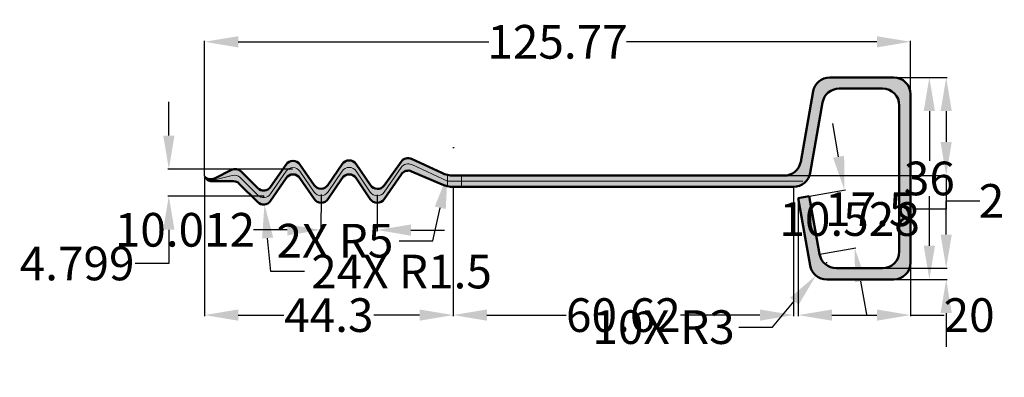
# Model space of a CAD drawing. Units: millimetres. Extents: x -64 to 111, y -49 to 15.
import ezdxf

# ---------------------------------------------------------------- set-up
doc = ezdxf.new("R2010")
doc.units = ezdxf.units.MM
doc.header["$MEASUREMENT"] = 0
doc.layers.add('M-DETL', color=251, linetype='Continuous', lineweight=18, true_color=0x636466)
doc.layers.add('M-HATC', color=251, linetype='Continuous', lineweight=18, true_color=0x636466)
doc.layers.add('M-DIMS', color=2, linetype='Continuous', lineweight=18)
doc.layers.add('M-OUTL', color=7, linetype='Continuous', lineweight=50)
doc.styles.get("Standard").update_dxf_attribs({"font": 'arial.ttf'})
doc.dimstyles.get("Standard").update_dxf_attribs({"dimtxt": 6, "dimasz": 6, "dimexe": 0.18, "dimexo": 0.0625, "dimgap": 0.09, "dimtad": 0, "dimtih": 1, "dimtoh": 1, "dimdec": 0, "dimzin": 0, "dimdsep": 46, "dimtxsty": 'Standard', "dimcen": 0.09, "dimadec": 0, "dimazin": 0, "dimtfac": 1, "dimtdec": 0, "dimtofl": 0, "dimtmove": 0, "dimatfit": 3, "dimfxl": 1, "dimtolj": 1, "dimtzin": 0, "dimarcsym": 0})

# ---------------------------------------------------------------- blocks, each defined once
blk = doc.blocks.new('*D1')
at = {"layer": 'Defpoints', "color": 0, "transparency": 16777216}
for p in [(94.41, 11.25), (94.41, 1.9), (-31.35, -12.77)]:
    blk.add_point(p, dxfattribs=at)
at = {"layer": 'M-DIMS', "color": 0, "lineweight": -2, "transparency": 16777216}
for p, q in [((-31.35, -12.71), (-31.35, 11.43)), ((-25.35, 11.25), (19.27, 11.25)), ((88.41, 11.25), (43.79, 11.25)), ((94.41, 1.97), (94.41, 11.43))]:
    blk.add_line(p, q, dxfattribs=at)
at = {"layer": 'M-DIMS', "color": 0, "transparency": 16777216}
for points in [[(-25.35, 12.25), (-25.35, 10.25), (-31.35, 11.25)], [(88.41, 12.25), (88.41, 10.25), (94.41, 11.25)]]:
    blk.add_solid(points, dxfattribs=at)
at = {"layer": 'M-DIMS', "color": 0, "transparency": 16777216, "insert": (31.53, 11.25), "char_height": 6, "attachment_point": 5}
blk.add_mtext('\\A1;125.77', dxfattribs=at)
blk = doc.blocks.new('*D2')
at = {"layer": 'Defpoints', "color": 0, "transparency": 16777216}
for p in [(91.41, 4.9), (91.41, -31.1), (97.76, -31.1)]:
    blk.add_point(p, dxfattribs=at)
at = {"layer": 'M-DIMS', "color": 0, "lineweight": -2, "transparency": 16777216}
for p, q in [((91.48, 4.9), (97.94, 4.9)), ((97.76, -1.1), (97.76, -9.94)), ((97.76, -25.1), (97.76, -16.25)), ((91.48, -31.1), (97.94, -31.1))]:
    blk.add_line(p, q, dxfattribs=at)
at = {"layer": 'M-DIMS', "color": 0, "transparency": 16777216}
for points in [[(96.76, -1.1), (98.76, -1.1), (97.76, 4.9)], [(96.76, -25.1), (98.76, -25.1), (97.76, -31.1)]]:
    blk.add_solid(points, dxfattribs=at)
at = {"layer": 'M-DIMS', "color": 0, "transparency": 16777216, "insert": (97.76, -13.1), "char_height": 6, "attachment_point": 5}
blk.add_mtext('\\A1;36', dxfattribs=at)
blk = doc.blocks.new('*D3')
at = {"layer": 'Defpoints', "color": 0, "transparency": 16777216}
for p in [(12.95, -14.6), (73.57, -14.6), (73.57, -37.45)]:
    blk.add_point(p, dxfattribs=at)
at = {"layer": 'M-DIMS', "color": 0, "lineweight": -2, "transparency": 16777216}
for p, q in [((12.95, -14.66), (12.95, -37.63)), ((73.57, -14.66), (73.57, -37.63)), ((18.95, -37.45), (33.06, -37.45)), ((67.57, -37.45), (53.46, -37.45))]:
    blk.add_line(p, q, dxfattribs=at)
at = {"layer": 'M-DIMS', "color": 0, "transparency": 16777216}
for points in [[(18.95, -36.45), (18.95, -38.45), (12.95, -37.45)], [(67.57, -36.45), (67.57, -38.45), (73.57, -37.45)]]:
    blk.add_solid(points, dxfattribs=at)
at = {"layer": 'M-DIMS', "color": 0, "transparency": 16777216, "insert": (43.26, -37.45), "char_height": 6, "attachment_point": 5}
blk.add_mtext('\\A1;60.62', dxfattribs=at)
blk = doc.blocks.new('*D4')
at = {"layer": 'Defpoints', "color": 0, "transparency": 16777216}
for p in [(74.41, -16.6), (94.41, -28.1), (94.41, -37.45)]:
    blk.add_point(p, dxfattribs=at)
at = {"layer": 'M-DIMS', "color": 0, "lineweight": -2, "transparency": 16777216}
for p, q in [((74.41, -16.66), (74.41, -37.63)), ((94.41, -28.16), (94.41, -37.63)), ((80.41, -37.45), (88.41, -37.45)), ((94.41, -37.45), (100.41, -37.45))]:
    blk.add_line(p, q, dxfattribs=at)
at = {"layer": 'M-DIMS', "color": 0, "transparency": 16777216}
for points in [[(80.41, -36.45), (80.41, -38.45), (74.41, -37.45)], [(88.41, -36.45), (88.41, -38.45), (94.41, -37.45)]]:
    blk.add_solid(points, dxfattribs=at)
at = {"layer": 'M-DIMS', "color": 0, "transparency": 16777216, "insert": (104.84, -37.45), "char_height": 6, "attachment_point": 5}
blk.add_mtext('\\A1;20', dxfattribs=at)
blk = doc.blocks.new('*D5')
at = {"layer": 'Defpoints', "color": 0, "transparency": 16777216}
for p in [(89.41, -29.1), (100.76, -29.1), (91.41, -31.1)]:
    blk.add_point(p, dxfattribs=at)
at = {"layer": 'M-DIMS', "color": 0, "lineweight": -2, "transparency": 16777216}
for p, q in [((100.76, -23.1), (100.76, -17.1)), ((100.76, -17.1), (106.76, -17.1)), ((89.48, -29.1), (100.94, -29.1)), ((91.48, -31.1), (100.94, -31.1)), ((100.76, -37.1), (100.76, -43.1))]:
    blk.add_line(p, q, dxfattribs=at)
at = {"layer": 'M-DIMS', "color": 0, "transparency": 16777216}
for points in [[(99.76, -23.1), (101.76, -23.1), (100.76, -29.1)], [(99.76, -37.1), (101.76, -37.1), (100.76, -31.1)]]:
    blk.add_solid(points, dxfattribs=at)
at = {"layer": 'M-DIMS', "color": 0, "transparency": 16777216, "insert": (108.84, -17.1), "char_height": 6, "attachment_point": 5}
blk.add_mtext('\\A1;2', dxfattribs=at)
blk = doc.blocks.new('*D6')
at = {"layer": 'Defpoints', "color": 0, "transparency": 16777216}
for p in [(91.41, 4.9), (71.9, -12.6), (100.76, -12.6)]:
    blk.add_point(p, dxfattribs=at)
at = {"layer": 'M-DIMS', "color": 0, "lineweight": -2, "transparency": 16777216}
for p, q in [((91.48, 4.9), (100.94, 4.9)), ((100.76, -1.1), (100.76, -6.6)), ((71.96, -12.6), (100.94, -12.6)), ((100.76, -12.6), (100.76, -18.6)), ((100.76, -18.6), (94.76, -18.6))]:
    blk.add_line(p, q, dxfattribs=at)
at = {"layer": 'M-DIMS', "color": 0, "transparency": 16777216}
for points in [[(99.76, -1.1), (101.76, -1.1), (100.76, 4.9)], [(99.76, -6.6), (101.76, -6.6), (100.76, -12.6)]]:
    blk.add_solid(points, dxfattribs=at)
at = {"layer": 'M-DIMS', "color": 0, "transparency": 16777216, "insert": (87.14, -18.6), "char_height": 6, "attachment_point": 5}
blk.add_mtext('\\A1;17.5', dxfattribs=at)
blk = doc.blocks.new('*D7')
at = {"layer": 'Defpoints', "color": 0, "transparency": 16777216}
for p in [(76.38, -16.25), (84.46, -25.51), (78.21, -26.62)]:
    blk.add_point(p, dxfattribs=at)
at = {"layer": 'M-DIMS', "color": 0, "lineweight": -2, "transparency": 16777216}
for p, q in [((81.59, -9.24), (80.55, -3.33)), ((76.44, -16.24), (82.81, -15.12)), ((78.27, -26.61), (84.64, -25.48)), ((85.51, -31.42), (86.55, -37.33))]:
    blk.add_line(p, q, dxfattribs=at)
at = {"layer": 'M-DIMS', "color": 0, "transparency": 16777216}
for points in [[(82.58, -9.06), (80.61, -9.41), (82.64, -15.15)], [(86.49, -31.25), (84.52, -31.6), (84.46, -25.51)]]:
    blk.add_solid(points, dxfattribs=at)
at = {"layer": 'M-DIMS', "color": 0, "transparency": 16777216, "insert": (83.55, -20.33), "char_height": 6, "attachment_point": 5}
blk.add_mtext('\\A1;10.528', dxfattribs=at)
blk = doc.blocks.new('*D8')
at = {"layer": 'Defpoints', "color": 0, "transparency": 16777216}
for p in [(-10.59, -15.92), (-0.57, -15.94), (-10.6, -22.27)]:
    blk.add_point(p, dxfattribs=at)
at = {"layer": 'M-DIMS', "color": 0, "lineweight": -2, "transparency": 16777216}
for p, q in [((-10.59, -15.98), (-10.6, -22.45)), ((-0.57, -16), (-0.59, -22.47)), ((-16.6, -22.26), (-22.6, -22.25)), ((5.41, -22.3), (11.41, -22.31))]:
    blk.add_line(p, q, dxfattribs=at)
at = {"layer": 'M-DIMS', "color": 0, "transparency": 16777216}
for points in [[(-16.6, -21.26), (-16.6, -23.26), (-10.6, -22.27)], [(5.42, -21.3), (5.41, -23.3), (-0.59, -22.29)]]:
    blk.add_solid(points, dxfattribs=at)
at = {"layer": 'M-DIMS', "color": 0, "transparency": 16777216, "insert": (-34.83, -22.25), "char_height": 6, "attachment_point": 5}
blk.add_mtext('\\A1;10.012', dxfattribs=at)
blk = doc.blocks.new('*D9')
at = {"layer": 'Defpoints', "color": 0, "transparency": 16777216}
for p in [(-31.35, -12.77), (12.95, -14.6), (12.95, -37.45)]:
    blk.add_point(p, dxfattribs=at)
at = {"layer": 'M-DIMS', "color": 0, "lineweight": -2, "transparency": 16777216}
for p, q in [((-31.35, -12.83), (-31.35, -37.63)), ((12.95, -14.66), (12.95, -37.63)), ((-25.35, -37.45), (-17.2, -37.45)), ((6.95, -37.45), (-1.2, -37.45))]:
    blk.add_line(p, q, dxfattribs=at)
at = {"layer": 'M-DIMS', "color": 0, "transparency": 16777216}
for points in [[(-25.35, -36.45), (-25.35, -38.45), (-31.35, -37.45)], [(6.95, -36.45), (6.95, -38.45), (12.95, -37.45)]]:
    blk.add_solid(points, dxfattribs=at)
at = {"layer": 'M-DIMS', "color": 0, "transparency": 16777216, "insert": (-9.2, -37.45), "char_height": 6, "attachment_point": 5}
blk.add_mtext('\\A1;44.3', dxfattribs=at)
blk = doc.blocks.new('*D10')
at = {"layer": 'Defpoints', "color": 0, "transparency": 16777216}
for p in [(-15.59, -11.45), (-37.7, -16.25), (-20.81, -16.25)]:
    blk.add_point(p, dxfattribs=at)
at = {"layer": 'M-DIMS', "color": 0, "lineweight": -2, "transparency": 16777216}
for p, q in [((-37.7, -5.45), (-37.7, 0.55)), ((-15.65, -11.45), (-37.88, -11.45)), ((-20.87, -16.25), (-37.88, -16.25)), ((-37.7, -22.25), (-37.7, -28.25)), ((-37.7, -28.25), (-43.7, -28.25))]:
    blk.add_line(p, q, dxfattribs=at)
at = {"layer": 'M-DIMS', "color": 0, "transparency": 16777216}
for points in [[(-38.7, -5.45), (-36.7, -5.45), (-37.7, -11.45)], [(-38.7, -22.25), (-36.7, -22.25), (-37.7, -16.25)]]:
    blk.add_solid(points, dxfattribs=at)
at = {"layer": 'M-DIMS', "color": 0, "transparency": 16777216, "insert": (-54.04, -28.25), "char_height": 6, "attachment_point": 5}
blk.add_mtext('\\A1;4.799', dxfattribs=at)
blk = doc.blocks.new('*D11')
at = {"layer": 'Defpoints', "color": 0, "transparency": 16777216}
for p in [(13.02, -7.6), (11.94, -12.48)]:
    blk.add_point(p, dxfattribs=at)
at = {"layer": 'M-DIMS', "color": 0, "lineweight": -2, "transparency": 16777216}
for p, q in [((12.93, -7.6), (13.11, -7.6)), ((13.02, -7.69), (13.02, -7.51)), ((9.34, -24.19), (10.64, -18.34)), ((3.34, -24.19), (9.34, -24.19))]:
    blk.add_line(p, q, dxfattribs=at)
at = {"layer": 'M-DIMS', "color": 0, "transparency": 16777216}
blk.add_solid([(9.66, -18.12), (11.62, -18.55), (11.94, -12.48)], dxfattribs=at)
at = {"layer": 'M-DIMS', "color": 0, "transparency": 16777216, "insert": (-8.11, -24.19), "char_height": 6, "attachment_point": 5}
blk.add_mtext('\\A1;2X R5', dxfattribs=at)
blk = doc.blocks.new('*D12')
at = {"layer": 'Defpoints', "color": 0, "transparency": 16777216}
for p in [(79.49, -28.1), (77.56, -30.39)]:
    blk.add_point(p, dxfattribs=at)
at = {"layer": 'M-DIMS', "color": 0, "lineweight": -2, "transparency": 16777216}
for p, q in [((79.49, -28.19), (79.49, -28.01)), ((79.4, -28.1), (79.58, -28.1)), ((69.85, -39.59), (73.7, -34.99)), ((63.85, -39.59), (69.85, -39.59))]:
    blk.add_line(p, q, dxfattribs=at)
at = {"layer": 'M-DIMS', "color": 0, "transparency": 16777216}
blk.add_solid([(72.94, -34.35), (74.47, -35.63), (77.56, -30.39)], dxfattribs=at)
at = {"layer": 'M-DIMS', "color": 0, "transparency": 16777216, "insert": (50.42, -39.59), "char_height": 6, "attachment_point": 5}
blk.add_mtext('\\A1;10X R3', dxfattribs=at)
blk = doc.blocks.new('*D13')
at = {"layer": 'Defpoints', "color": 0, "transparency": 16777216}
for p in [(-20.81, -16.25), (-20.67, -17.74)]:
    blk.add_point(p, dxfattribs=at)
at = {"layer": 'M-DIMS', "color": 0, "lineweight": -2, "transparency": 16777216}
for p, q in [((-20.9, -16.25), (-20.72, -16.25)), ((-20.81, -16.34), (-20.81, -16.16)), ((-19.53, -29.69), (-20.1, -23.72)), ((-13.53, -29.69), (-19.53, -29.69))]:
    blk.add_line(p, q, dxfattribs=at)
at = {"layer": 'M-DIMS', "color": 0, "transparency": 16777216}
blk.add_solid([(-19.1, -23.62), (-21.09, -23.81), (-20.67, -17.74)], dxfattribs=at)
at = {"layer": 'M-DIMS', "color": 0, "transparency": 16777216, "insert": (3.75, -29.69), "char_height": 6, "attachment_point": 5}
blk.add_mtext('\\A1;24X R1.5', dxfattribs=at)

msp = doc.modelspace()

# ---------------------------------------------------------------- hatches: boundary and pattern name
at = {"layer": 'M-HATC'}
h = msp.add_hatch(color=256, dxfattribs=at)
h.dxf.hatch_style = 1
h.set_gradient(color1=(248, 215, 49), color2=(248, 246, 176), tint=1)
h.paths.add_polyline_path([(-14.3494, -10.6033, 0.52714571), (-16.8245, -10.6033), (-19.5662, -14.606, -0.4694537), (-21.8644, -14.8191), (-24.8225, -11.8609, 0.32282281), (-26.554, -11.5799), (-29.5807, -13.0933, -0.31146656), (-31.2675, -12.8552, 0.29508116), (-29.7261, -13.3812), (-26.4109, -12.5524, -0.26344714), (-24.9864, -12.947), (-21.8685, -16.0649, 0.47042379), (-19.5676, -15.848), (-16.8272, -11.8196, -0.52917824), (-14.3467, -11.8196), (-11.8314, -15.5171, 0.53018636), (-9.3483, -15.5132), (-6.8299, -11.7859, -0.53119533), (-4.3441, -11.7859), (-1.8172, -15.5257, 0.52814262), (0.6605, -15.5376), (3.693, -11.1404, -0.36606977), (5.5622, -10.6327), (11.913, -13.5964), (14.413, -13.5964), (14.413, -12.5964), (13.0223, -12.5964, -0.10959241), (10.9078, -12.1274), (5.5431, -9.6238, 0.36139898), (3.6882, -10.1112), (0.6678, -14.3397, -0.5228784), (-1.7956, -14.3076), (-4.3441, -10.5359, 0.53119533), (-6.8299, -10.5359), (-9.3525, -14.2695, -0.52916882), (-11.833, -14.2773)])
h.paths.add_polyline_path([(-14.3467, -11.8196, 0.52917824), (-16.8272, -11.8196), (-19.5676, -15.848, -0.47042379), (-21.8685, -16.0649), (-24.9864, -12.947, 0.26344714), (-26.4109, -12.5524), (-29.7261, -13.3812, -0.25291889), (-31.1079, -13.0277, 0.22913347), (-29.932, -13.5964), (-26.2083, -13.5964, -0.19891237), (-25.1476, -14.0358), (-21.8726, -17.3108, 0.47138562), (-19.5691, -17.0899), (-16.8299, -13.0359, -0.53119533), (-14.3441, -13.0359), (-11.8299, -16.757, 0.53119533), (-9.3441, -16.757), (-6.8299, -13.0359, -0.53119533), (-4.3441, -13.0359), (-1.8175, -16.7753, 0.52821281), (0.6604, -16.7869), (3.7128, -12.3588, -0.35840084), (5.5448, -11.834), (10.961, -14.1835, 0.0500968), (11.913, -14.4876), (11.913, -13.5964), (5.5622, -10.6327, 0.36606977), (3.693, -11.1404), (0.6605, -15.5376, -0.52814262), (-1.8172, -15.5257), (-4.3441, -11.7859, 0.53119533), (-6.8299, -11.7859), (-9.3483, -15.5132, -0.53018636), (-11.8314, -15.5171)])
h.paths.add_polyline_path([(14.413, -13.5964), (11.913, -13.5964), (11.913, -14.4876, 0.05231524), (12.9508, -14.5964), (14.413, -14.5964)], flags=17)
h.paths.add_polyline_path([(76.5283, -12.1174), (78.7398, 0.4245, -0.36397023), (81.6942, 2.9036), (89.4137, 2.9036, -0.41421356), (92.4137, -0.0964), (92.4137, -26.0964, -0.41421356), (89.4137, -29.0964), (81.1653, -29.0964, -0.36397023), (78.2108, -26.6174), (76.3826, -16.2491), (74.413, -16.5964), (76.5326, -28.6174, 0.36397023), (79.4871, -31.0964), (91.4137, -31.0964, 0.41421356), (94.4137, -28.0964), (94.4137, 1.9036, 0.41421356), (91.4137, 4.9036), (80.016, 4.9036, 0.36397023), (77.0616, 2.4245), (74.8501, -10.1174, -0.36397023), (71.8957, -12.5964), (14.413, -12.5964), (14.413, -13.5964), (14.413, -14.5964), (73.5739, -14.5964, 0.36397023)])

# ---------------------------------------------------------------- linework, layer by layer
at = {"layer": 'M-DETL'}
for p, q in [((-16.8272, -11.8196), (-19.5676, -15.848)), ((-11.8314, -15.5171), (-14.3467, -11.8196)), ((-6.8299, -11.7859), (-9.3483, -15.5132)), ((-1.8172, -15.5257), (-4.3441, -11.7859)), ((3.693, -11.1404), (0.6605, -15.5376)), ((11.913, -13.5964), (5.5622, -10.6327)), ((-26.2083, -13.5964), (-29.932, -13.5964)), ((-26.4109, -12.5524), (-29.7261, -13.3812)), ((-21.8685, -16.0649), (-24.9864, -12.947)), ((11.913, -13.5964), (11.913, -12.5964)), ((11.913, -13.4977), (11.913, -14.4977)), ((11.913, -13.5964), (14.413, -13.5964)), ((14.413, -12.5964), (14.413, -14.5964)), ((75.2521, -13.5964), (14.413, -13.5964))]:
    msp.add_line(p, q, dxfattribs=at)
for centre, start, end in [((4.9279, -11.992), 64.983107, 145.407711), ((-15.587, -12.6633), 34.226362, 145.773638), ((-5.587, -12.6257), 34.045937, 145.954063), ((-30.0899, -11.926), 218.274897, 284.036243), ((-26.0471, -14.0076), 45, 104.036243), ((-10.5912, -14.6734), 214.226362, 325.954063), ((-0.5743, -14.686), 214.045937, 325.407711), ((-20.8078, -15.0043), 225, 325.773638)]:
    msp.add_arc(centre, 1.5, start, end, dxfattribs=at)
at = {"layer": 'M-OUTL'}
for p, q in [((91.4137, 4.9036), (80.016, 4.9036)), ((74.8501, -10.1174), (77.0616, 2.4245)), ((81.6942, 2.9036), (89.4137, 2.9036)), ((94.4137, 1.9036), (94.4137, -28.0964)), ((76.5283, -12.1174), (78.7398, 0.4245)), ((92.4137, -0.0964), (92.4137, -26.0964)), ((3.6882, -10.1112), (0.6678, -14.3397)), ((10.9078, -12.1274), (5.5431, -9.6238)), ((-26.554, -11.5799), (-29.5807, -13.0933)), ((-21.8644, -14.8191), (-24.8225, -11.8609)), ((-16.8245, -10.6033), (-19.5662, -14.606)), ((-11.833, -14.2773), (-14.3494, -10.6033)), ((-6.8299, -10.5359), (-9.3525, -14.2695)), ((-1.7956, -14.3076), (-4.3441, -10.5359)), ((10.961, -14.1835), (5.5448, -11.834)), ((-31.0322, -13.116), (-31.0576, -13.0885)), ((-26.2083, -13.5964), (-29.932, -13.5964)), ((-16.8299, -13.0359), (-19.5691, -17.0899)), ((-11.8299, -16.757), (-14.3441, -13.0359)), ((-6.8299, -13.0359), (-9.3441, -16.757)), ((-1.8175, -16.7753), (-4.3441, -13.0359)), ((3.7128, -12.3588), (0.6604, -16.7869)), ((14.413, -12.5964), (13.0223, -12.5964)), ((14.413, -12.5964), (71.8957, -12.5964)), ((-21.8726, -17.3108), (-25.1476, -14.0358)), ((14.413, -14.5964), (12.9508, -14.5964)), ((14.413, -14.5964), (73.5739, -14.5964)), ((74.413, -16.5964), (76.3826, -16.2491)), ((74.413, -16.5964), (76.5326, -28.6174)), ((76.3826, -16.2491), (78.2108, -26.6174)), ((81.1653, -29.0964), (89.4137, -29.0964)), ((79.4871, -31.0964), (91.4137, -31.0964))]:
    msp.add_line(p, q, dxfattribs=at)
for centre, radius, start, end in [((80.016, 1.9036), 3, 90, 170), ((91.4137, 1.9036), 3, 0, 90), ((81.6942, -0.0964), 3, 90, 170), ((89.4137, -0.0964), 3, 0, 90), ((-15.587, -11.4509), 1.5, 34.408472, 145.591528), ((-5.587, -11.3757), 1.5, 34.045937, 145.954063), ((4.9088, -10.9831), 1.5, 64.983107, 144.462322), ((71.8957, -9.5964), 3, 270, 350), ((-25.8832, -12.9216), 1.5, 45, 116.565051), ((4.9479, -13.2101), 1.5, 66.5494, 145.42029), ((13.0223, -7.5964), 5, 244.983107, 270), ((73.5739, -11.5964), 3, 270, 350), ((-30.2515, -11.7516), 1.5, 222.819844, 296.565051), ((-29.932, -12.0964), 1.5, 218.377593, 270), ((-26.2083, -15.0964), 1.5, 45, 90), ((-15.587, -13.8757), 1.5, 34.045937, 145.954063), ((-5.587, -13.8757), 1.5, 34.045937, 145.954063), ((-20.8037, -13.7584), 1.5, 225, 325.591528), ((-10.5954, -13.4297), 1.5, 214.408472, 325.954063), ((-0.5528, -13.4678), 1.5, 214.045937, 324.462322), ((12.9508, -9.5964), 5, 246.5494, 270), ((-20.812, -16.2501), 1.5, 225, 325.954063), ((-10.587, -15.9172), 1.5, 214.045937, 325.954063), ((-0.5746, -15.9355), 1.5, 214.045937, 325.42029), ((89.4137, -26.0964), 3, 270, 0), ((81.1653, -26.0964), 3, 190, 270), ((79.4871, -28.0964), 3, 190, 270), ((91.4137, -28.0964), 3, 270, 0)]:
    msp.add_arc(centre, radius, start, end, dxfattribs=at)

# ---------------------------------------------------------------- dimensions: what is measured, and where the dimension line sits
at = {"layer": 'M-DIMS'}
for base, p1, p2, override, picture, middle in [((94.4137, 11.2536), (-31.3517, -12.7712), (94.4137, 1.9036), {"dimdec": 2, "dimlfac": 1, "dimrnd": 0, "dimzin": 0, "dimdsep": 46, "dimlunit": 2}, '*D1', (31.531, 11.2536)), ((12.9508, -37.4464), (-31.3517, -12.7712), (12.9508, -14.5964), {"dimdec": 1, "dimlfac": 1, "dimrnd": 0, "dimzin": 0, "dimdsep": 46, "dimlunit": 2}, '*D9', (-9.2005, -37.4464)), ((73.5739, -37.4464), (12.9508, -14.5964), (73.5739, -14.5964), {"dimdec": 2, "dimlfac": 1, "dimrnd": 0, "dimzin": 0, "dimdsep": 46, "dimlunit": 2}, '*D3', (43.2623, -37.4464)), ((94.4137, -37.4464), (74.413, -16.5964), (94.4137, -28.0964), {"dimdec": 0, "dimlfac": 1, "dimrnd": 0, "dimzin": 0, "dimdsep": 46, "dimlunit": 2}, '*D4', (104.8421, -37.4464))]:
    dim = msp.add_linear_dim(base=base, p1=p1, p2=p2, dimstyle='Standard', override=override, dxfattribs=at)
    dim.commit()
    dim.dimension.update_dxf_attribs({"geometry": picture, "text_midpoint": middle})
for base, p1, p2, angle, override, picture, middle in [((100.7637, -12.5964), (91.4137, 4.9036), (71.8957, -12.5964), 90, {"dimdec": 1, "dimlfac": 1, "dimrnd": 0, "dimzin": 0, "dimdsep": 46, "dimlunit": 2}, '*D6', (87.141, -18.5964)), ((97.7637, -31.0964), (91.4137, 4.9036), (91.4137, -31.0964), 270, {"dimdec": 0, "dimlfac": 1, "dimrnd": 0, "dimzin": 0, "dimdsep": 46, "dimlunit": 2}, '*D2', (97.7637, -13.0964)), ((-37.7017, -16.2501), (-15.587, -11.4509), (-20.812, -16.2501), 90, {"dimdec": 3, "dimlfac": 1, "dimrnd": 0, "dimzin": 0, "dimdsep": 46, "dimlunit": 2}, '*D10', (-54.0421, -28.2501)), ((84.4644, -25.5147), (76.3826, -16.2491), (78.2108, -26.6174), 280, {"dimdec": 3, "dimlfac": 1, "dimrnd": 0, "dimzin": 0, "dimdsep": 46, "dimlunit": 2}, '*D7', (83.5503, -20.3306)), ((100.7637, -29.0964), (91.4137, -31.0964), (89.4137, -29.0964), 90, {"dimdec": 0, "dimlfac": 1, "dimrnd": 0, "dimzin": 0, "dimdsep": 46, "dimlunit": 2}, '*D5', (108.8408, -17.0964)), ((-10.5986, -22.2672), (-0.5746, -15.9355), (-10.587, -15.9172), 179.895026, {"dimdec": 3, "dimlfac": 1, "dimrnd": 0, "dimzin": 0, "dimdsep": 46, "dimlunit": 2}, '*D8', (-34.8298, -22.2452))]:
    dim = msp.add_linear_dim(base=base, p1=p1, p2=p2, angle=angle, dimstyle='Standard', override=override, dxfattribs=at)
    dim.commit()
    dim.dimension.update_dxf_attribs({"geometry": picture, "text_midpoint": middle})
for center, mpoint, text, override, picture, middle in [((13.0223, -7.5964), (11.9391, -12.4777), '2X <>', {"dimdec": 0, "dimlfac": 1, "dimrnd": 0, "dimzin": 0, "dimdsep": 46, "dimlunit": 2}, '*D11', (-8.108, -24.1927)), ((-20.812, -16.2501), (-20.669, -17.7433), '24X <>', {"dimdec": 1, "dimlfac": 1, "dimrnd": 0, "dimzin": 0, "dimdsep": 46, "dimlunit": 2}, '*D13', (3.7484, -29.6887)), ((79.4871, -28.0964), (77.5591, -30.3949), '10X <>', {"dimdec": 0, "dimlfac": 1, "dimrnd": 0, "dimzin": 0, "dimdsep": 46, "dimlunit": 2}, '*D12', (50.425, -39.5887))]:
    dim = msp.add_radius_dim(center=center, mpoint=mpoint, text=text, dimstyle='Standard', override=override, dxfattribs=at)
    dim.commit()
    dim.dimension.update_dxf_attribs({"geometry": picture, "text_midpoint": middle})

doc.saveas('drawing.dxf')
